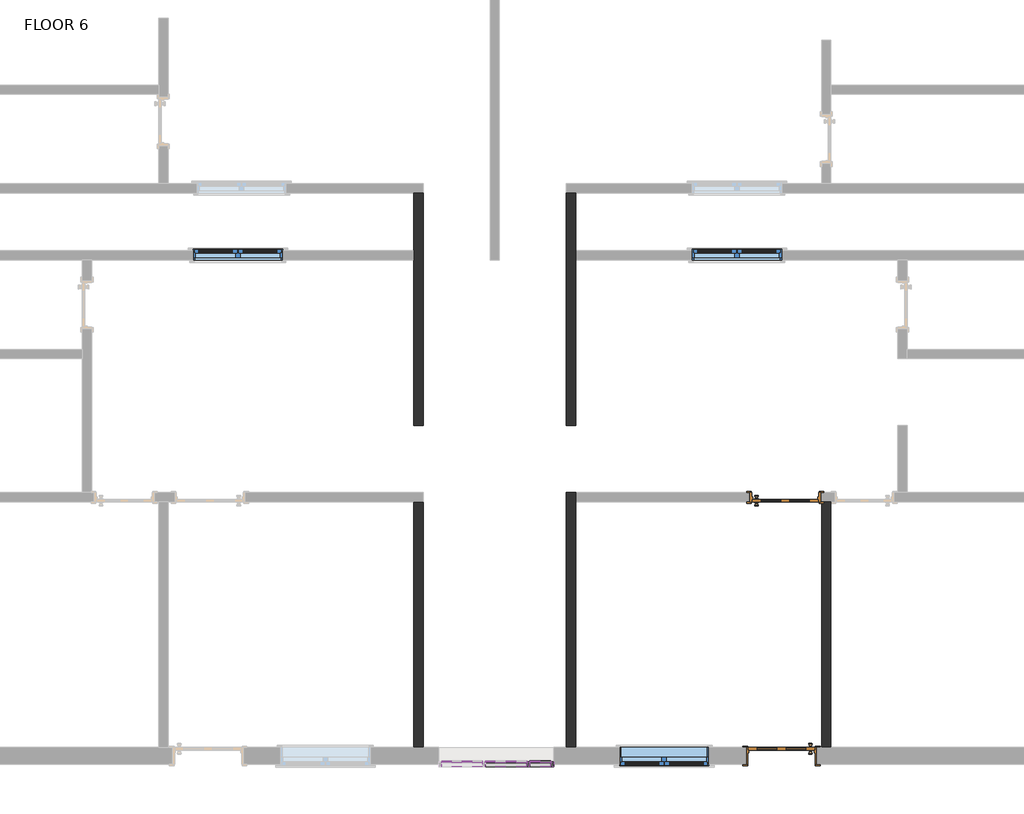
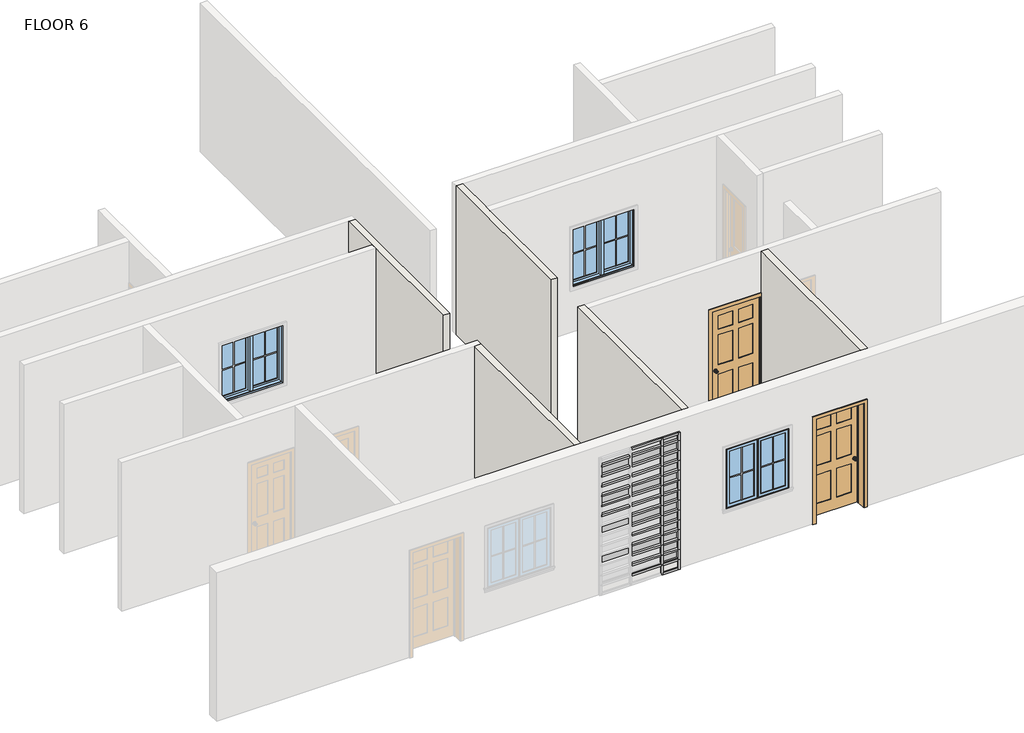
# One storey, part 2 of 4: 63 members, 22 plates, 5 walls, 3 windows, 2 doors.
"""IFC4 building model written with IfcOpenShell, lengths in millimetres."""

from ifc_helpers import new_model, si_unit, frame, origin, place, context, project, spatial, polyline, outline, extrude, faceted_brep, transform, mapped, element, save
from components import door_c610b25b, door_c5239341, member_56b223d9, member_a59c64b1, member_06854975, member_6a7c88b6, member_b8e7570c, member_a67f877f, member_00eacae2, member_ff422208, member_dc11c383, system_panel_glazed_b3845325, system_panel_glazed_23b8b45c, system_panel_glazed_58d257f9, system_panel_glazed_e426d894, system_panel_glazed_822b3193, window_9200f5ac, window_c2c97eee

model = new_model("IFC4")

# Units and contexts
model_context = context("Model", 3, world=origin())
ifc_project = project(units=[si_unit("LENGTHUNIT", "METRE", prefix="MILLI")], contexts=[model_context])

# Site, building, storey
site = spatial("IfcSite", under=ifc_project)
building = spatial("IfcBuilding", under=site)
storey = spatial("IfcBuildingStorey", under=building, Name="FLOOR 6", Elevation=9544.3725604)

# Doors
placement = place(None, origin())
door_shape = door_c610b25b(model_context)
element("IfcDoor", 1, ObjectType="Door-Interior-Single-6_Panel-Wood : 36\" x 84\"", at=placement, inside=storey, context=model_context, shape_type="MappedRepresentation", body=[
    mapped(door_shape, transform((-301.9137331, -4180.7343836, 9544.3725604), x_axis=(1.0, 0.0, 0.0), y_axis=(0.0, 1.0, 0.0), z_axis=(0.0, 0.0, 1.0))),
])
door_2_shape = door_c5239341(model_context)
element("IfcDoor", 2, ObjectType="Door-Interior-Single-6_Panel-Wood : 36\" x 84\"", at=placement, inside=storey, context=model_context, shape_type="MappedRepresentation", body=[
    mapped(door_2_shape, transform((-352.7137331, -7704.9843836, 9544.3725604), x_axis=(-1.0, 0.0, 0.0), y_axis=(0.0, -1.0, 0.0), z_axis=(0.0, 0.0, 1.0))),
])

# Members
member_shape = member_56b223d9(model_context)
element("IfcMember", 3, ObjectType="Rectangular Mullion : 1.5\" x 2.5\" rectangular", at=placement, inside=storey, context=model_context, shape_type="MappedRepresentation", body=[
    mapped(member_shape, transform((-3807.0334597, -7822.4593836, 9544.3725604), x_axis=(1.0, 0.0, 0.0), y_axis=(0.0, -1.0, 0.0), z_axis=(0.0, 0.0, -1.0))),
])
element("IfcMember", 4, ObjectType="Rectangular Mullion : 1.5\" x 2.5\" rectangular", at=placement, inside=storey, context=model_context, shape_type="MappedRepresentation", body=[
    mapped(member_shape, transform((-3807.0334597, -7822.4593836, 9747.5725604), x_axis=(1.0, 0.0, 0.0), y_axis=(0.0, -1.0, 0.0), z_axis=(0.0, 0.0, -1.0))),
])
element("IfcMember", 5, ObjectType="Rectangular Mullion : 1.5\" x 2.5\" rectangular", at=placement, inside=storey, context=model_context, shape_type="MappedRepresentation", body=[
    mapped(member_shape, transform((-3807.0334597, -7822.4593836, 9950.7725604), x_axis=(1.0, 0.0, 0.0), y_axis=(0.0, -1.0, 0.0), z_axis=(0.0, 0.0, -1.0))),
])
element("IfcMember", 6, ObjectType="Rectangular Mullion : 1.5\" x 2.5\" rectangular", at=placement, inside=storey, context=model_context, shape_type="MappedRepresentation", body=[
    mapped(member_shape, transform((-3807.0334597, -7822.4593836, 10153.9725604), x_axis=(1.0, 0.0, 0.0), y_axis=(0.0, -1.0, 0.0), z_axis=(0.0, 0.0, -1.0))),
])
element("IfcMember", 7, ObjectType="Rectangular Mullion : 1.5\" x 2.5\" rectangular", at=placement, inside=storey, context=model_context, shape_type="MappedRepresentation", body=[
    mapped(member_shape, transform((-3807.0334597, -7822.4593836, 10357.1725604), x_axis=(1.0, 0.0, 0.0), y_axis=(0.0, -1.0, 0.0), z_axis=(0.0, 0.0, -1.0))),
])
element("IfcMember", 8, ObjectType="Rectangular Mullion : 1.5\" x 2.5\" rectangular", at=placement, inside=storey, context=model_context, shape_type="MappedRepresentation", body=[
    mapped(member_shape, transform((-3807.0334597, -7822.4593836, 10560.3725604), x_axis=(1.0, 0.0, 0.0), y_axis=(0.0, -1.0, 0.0), z_axis=(0.0, 0.0, -1.0))),
])
element("IfcMember", 9, ObjectType="Rectangular Mullion : 1.5\" x 2.5\" rectangular", at=placement, inside=storey, context=model_context, shape_type="MappedRepresentation", body=[
    mapped(member_shape, transform((-3807.0334597, -7822.4593836, 10763.5725604), x_axis=(1.0, 0.0, 0.0), y_axis=(0.0, -1.0, 0.0), z_axis=(0.0, 0.0, -1.0))),
])
element("IfcMember", 10, ObjectType="Rectangular Mullion : 1.5\" x 2.5\" rectangular", at=placement, inside=storey, context=model_context, shape_type="MappedRepresentation", body=[
    mapped(member_shape, transform((-3807.0334597, -7822.4593836, 10966.7725604), x_axis=(1.0, 0.0, 0.0), y_axis=(0.0, -1.0, 0.0), z_axis=(0.0, 0.0, -1.0))),
])
element("IfcMember", 11, ObjectType="Rectangular Mullion : 1.5\" x 2.5\" rectangular", at=placement, inside=storey, context=model_context, shape_type="MappedRepresentation", body=[
    mapped(member_shape, transform((-3807.0334597, -7822.4593836, 11169.9725604), x_axis=(1.0, 0.0, 0.0), y_axis=(0.0, -1.0, 0.0), z_axis=(0.0, 0.0, -1.0))),
])
element("IfcMember", 12, ObjectType="Rectangular Mullion : 1.5\" x 2.5\" rectangular", at=placement, inside=storey, context=model_context, shape_type="MappedRepresentation", body=[
    mapped(member_shape, transform((-3807.0334597, -7822.4593836, 11373.1725604), x_axis=(1.0, 0.0, 0.0), y_axis=(0.0, -1.0, 0.0), z_axis=(0.0, 0.0, -1.0))),
])
element("IfcMember", 13, ObjectType="Rectangular Mullion : 1.5\" x 2.5\" rectangular", at=placement, inside=storey, context=model_context, shape_type="MappedRepresentation", body=[
    mapped(member_shape, transform((-3807.0334597, -7822.4593836, 11576.3725604), x_axis=(1.0, 0.0, 0.0), y_axis=(0.0, -1.0, 0.0), z_axis=(0.0, 0.0, -1.0))),
])
element("IfcMember", 14, ObjectType="Rectangular Mullion : 1.5\" x 2.5\" rectangular", at=placement, inside=storey, context=model_context, shape_type="MappedRepresentation", body=[
    mapped(member_shape, transform((-3807.0334597, -7822.4593836, 11779.5725604), x_axis=(1.0, 0.0, 0.0), y_axis=(0.0, -1.0, 0.0), z_axis=(0.0, 0.0, -1.0))),
])
element("IfcMember", 15, ObjectType="Rectangular Mullion : 1.5\" x 2.5\" rectangular", at=placement, inside=storey, context=model_context, shape_type="MappedRepresentation", body=[
    mapped(member_shape, transform((-3807.0334597, -7822.4593836, 11982.7725604), x_axis=(1.0, 0.0, 0.0), y_axis=(0.0, -1.0, 0.0), z_axis=(0.0, 0.0, -1.0))),
])
member_2_shape = member_a59c64b1(model_context)
element("IfcMember", 16, ObjectType="Rectangular Mullion : 1.5\" x 2.5\" rectangular", at=placement, inside=storey, context=model_context, shape_type="MappedRepresentation", body=[
    mapped(member_2_shape, transform((-3807.0334597, -7822.4593836, 12185.9725604), x_axis=(1.0, 0.0, 0.0), y_axis=(0.0, -1.0, 0.0), z_axis=(0.0, 0.0, -1.0))),
])
member_3_shape = member_06854975(model_context)
element("IfcMember", 17, ObjectType="Rectangular Mullion : 1.5\" x 2.5\" rectangular", at=placement, inside=storey, context=model_context, shape_type="MappedRepresentation", body=[
    mapped(member_3_shape, transform((-3499.7513929, -7822.4593836, 12351.7551755), x_axis=(0.0, 0.0, 1.0), y_axis=(0.0, -1.0, 0.0), z_axis=(1.0, 0.0, 0.0))),
])
member_4_shape = member_6a7c88b6(model_context)
element("IfcMember", 18, ObjectType="Rectangular Mullion : 1.5\" x 2.5\" rectangular", at=placement, inside=storey, context=model_context, shape_type="MappedRepresentation", body=[
    mapped(member_4_shape, transform((-4435.6834597, -7822.4593836, 11169.9725604), x_axis=(0.0, 0.0, 1.0), y_axis=(0.0, -1.0, 0.0), z_axis=(1.0, 0.0, 0.0))),
])
element("IfcMember", 19, ObjectType="Rectangular Mullion : 1.5\" x 2.5\" rectangular", at=placement, inside=storey, context=model_context, shape_type="MappedRepresentation", body=[
    mapped(member_4_shape, transform((-4435.6834597, -7822.4593836, 11373.1725604), x_axis=(0.0, 0.0, 1.0), y_axis=(0.0, -1.0, 0.0), z_axis=(1.0, 0.0, 0.0))),
])
element("IfcMember", 20, ObjectType="Rectangular Mullion : 1.5\" x 2.5\" rectangular", at=placement, inside=storey, context=model_context, shape_type="MappedRepresentation", body=[
    mapped(member_4_shape, transform((-4435.6834597, -7822.4593836, 11576.3725604), x_axis=(0.0, 0.0, 1.0), y_axis=(0.0, -1.0, 0.0), z_axis=(1.0, 0.0, 0.0))),
])
element("IfcMember", 21, ObjectType="Rectangular Mullion : 1.5\" x 2.5\" rectangular", at=placement, inside=storey, context=model_context, shape_type="MappedRepresentation", body=[
    mapped(member_4_shape, transform((-4435.6834597, -7822.4593836, 11779.5725604), x_axis=(0.0, 0.0, 1.0), y_axis=(0.0, -1.0, 0.0), z_axis=(1.0, 0.0, 0.0))),
])
element("IfcMember", 22, ObjectType="Rectangular Mullion : 1.5\" x 2.5\" rectangular", at=placement, inside=storey, context=model_context, shape_type="MappedRepresentation", body=[
    mapped(member_4_shape, transform((-4435.6834597, -7822.4593836, 11982.7725604), x_axis=(0.0, 0.0, 1.0), y_axis=(0.0, -1.0, 0.0), z_axis=(1.0, 0.0, 0.0))),
])
element("IfcMember", 23, ObjectType="Rectangular Mullion : 1.5\" x 2.5\" rectangular", at=placement, inside=storey, context=model_context, shape_type="MappedRepresentation", body=[
    mapped(member_4_shape, transform((-4435.6834597, -7822.4593836, 12185.9725604), x_axis=(0.0, 0.0, 1.0), y_axis=(0.0, -1.0, 0.0), z_axis=(1.0, 0.0, 0.0))),
])
member_5_shape = member_b8e7570c(model_context)
element("IfcMember", 24, ObjectType="Rectangular Mullion : 1.5\" x 2.5\" rectangular", at=placement, inside=storey, context=model_context, shape_type="MappedRepresentation", body=[
    mapped(member_5_shape, transform((-3826.0834597, -7822.4593836, 9747.5725604), x_axis=(0.0, 0.0, 1.0), y_axis=(0.0, -1.0, 0.0), z_axis=(1.0, 0.0, 0.0))),
])
element("IfcMember", 25, ObjectType="Rectangular Mullion : 1.5\" x 2.5\" rectangular", at=placement, inside=storey, context=model_context, shape_type="MappedRepresentation", body=[
    mapped(member_5_shape, transform((-3826.0834597, -7822.4593836, 9950.7725604), x_axis=(0.0, 0.0, 1.0), y_axis=(0.0, -1.0, 0.0), z_axis=(1.0, 0.0, 0.0))),
])
element("IfcMember", 26, ObjectType="Rectangular Mullion : 1.5\" x 2.5\" rectangular", at=placement, inside=storey, context=model_context, shape_type="MappedRepresentation", body=[
    mapped(member_5_shape, transform((-3826.0834597, -7822.4593836, 10153.9725604), x_axis=(0.0, 0.0, 1.0), y_axis=(0.0, -1.0, 0.0), z_axis=(1.0, 0.0, 0.0))),
])
element("IfcMember", 27, ObjectType="Rectangular Mullion : 1.5\" x 2.5\" rectangular", at=placement, inside=storey, context=model_context, shape_type="MappedRepresentation", body=[
    mapped(member_5_shape, transform((-3826.0834597, -7822.4593836, 10357.1725604), x_axis=(0.0, 0.0, 1.0), y_axis=(0.0, -1.0, 0.0), z_axis=(1.0, 0.0, 0.0))),
])
element("IfcMember", 28, ObjectType="Rectangular Mullion : 1.5\" x 2.5\" rectangular", at=placement, inside=storey, context=model_context, shape_type="MappedRepresentation", body=[
    mapped(member_5_shape, transform((-3826.0834597, -7822.4593836, 10560.3725604), x_axis=(0.0, 0.0, 1.0), y_axis=(0.0, -1.0, 0.0), z_axis=(1.0, 0.0, 0.0))),
])
element("IfcMember", 29, ObjectType="Rectangular Mullion : 1.5\" x 2.5\" rectangular", at=placement, inside=storey, context=model_context, shape_type="MappedRepresentation", body=[
    mapped(member_5_shape, transform((-3826.0834597, -7822.4593836, 10763.5725604), x_axis=(0.0, 0.0, 1.0), y_axis=(0.0, -1.0, 0.0), z_axis=(1.0, 0.0, 0.0))),
])
element("IfcMember", 30, ObjectType="Rectangular Mullion : 1.5\" x 2.5\" rectangular", at=placement, inside=storey, context=model_context, shape_type="MappedRepresentation", body=[
    mapped(member_5_shape, transform((-3826.0834597, -7822.4593836, 10966.7725604), x_axis=(0.0, 0.0, 1.0), y_axis=(0.0, -1.0, 0.0), z_axis=(1.0, 0.0, 0.0))),
])
element("IfcMember", 31, ObjectType="Rectangular Mullion : 1.5\" x 2.5\" rectangular", at=placement, inside=storey, context=model_context, shape_type="MappedRepresentation", body=[
    mapped(member_5_shape, transform((-3826.0834597, -7822.4593836, 11169.9725604), x_axis=(0.0, 0.0, 1.0), y_axis=(0.0, -1.0, 0.0), z_axis=(1.0, 0.0, 0.0))),
])
element("IfcMember", 32, ObjectType="Rectangular Mullion : 1.5\" x 2.5\" rectangular", at=placement, inside=storey, context=model_context, shape_type="MappedRepresentation", body=[
    mapped(member_5_shape, transform((-3826.0834597, -7822.4593836, 11373.1725604), x_axis=(0.0, 0.0, 1.0), y_axis=(0.0, -1.0, 0.0), z_axis=(1.0, 0.0, 0.0))),
])
element("IfcMember", 33, ObjectType="Rectangular Mullion : 1.5\" x 2.5\" rectangular", at=placement, inside=storey, context=model_context, shape_type="MappedRepresentation", body=[
    mapped(member_5_shape, transform((-3826.0834597, -7822.4593836, 11576.3725604), x_axis=(0.0, 0.0, 1.0), y_axis=(0.0, -1.0, 0.0), z_axis=(1.0, 0.0, 0.0))),
])
element("IfcMember", 34, ObjectType="Rectangular Mullion : 1.5\" x 2.5\" rectangular", at=placement, inside=storey, context=model_context, shape_type="MappedRepresentation", body=[
    mapped(member_5_shape, transform((-3826.0834597, -7822.4593836, 11779.5725604), x_axis=(0.0, 0.0, 1.0), y_axis=(0.0, -1.0, 0.0), z_axis=(1.0, 0.0, 0.0))),
])
element("IfcMember", 35, ObjectType="Rectangular Mullion : 1.5\" x 2.5\" rectangular", at=placement, inside=storey, context=model_context, shape_type="MappedRepresentation", body=[
    mapped(member_5_shape, transform((-3826.0834597, -7822.4593836, 11982.7725604), x_axis=(0.0, 0.0, 1.0), y_axis=(0.0, -1.0, 0.0), z_axis=(1.0, 0.0, 0.0))),
])
element("IfcMember", 36, ObjectType="Rectangular Mullion : 1.5\" x 2.5\" rectangular", at=placement, inside=storey, context=model_context, shape_type="MappedRepresentation", body=[
    mapped(member_5_shape, transform((-3826.0834597, -7822.4593836, 12185.9725604), x_axis=(0.0, 0.0, 1.0), y_axis=(0.0, -1.0, 0.0), z_axis=(1.0, 0.0, 0.0))),
])
member_6_shape = member_a67f877f(model_context)
element("IfcMember", 37, ObjectType="Rectangular Mullion : 1.5\" x 2.5\" rectangular", at=placement, inside=storey, context=model_context, shape_type="MappedRepresentation", body=[
    mapped(member_6_shape, transform((-3826.0834597, -7822.4593836, 12351.7551755), x_axis=(0.0, 0.0, 1.0), y_axis=(0.0, -1.0, 0.0), z_axis=(1.0, 0.0, 0.0))),
])
element("IfcMember", 38, ObjectType="Rectangular Mullion : 1.5\" x 2.5\" rectangular", at=placement, inside=storey, context=model_context, shape_type="MappedRepresentation", body=[
    mapped(member_3_shape, transform((-3787.9834597, -7822.4593836, 9544.3725604), x_axis=(0.0, 0.0, -1.0), y_axis=(0.0, -1.0, 0.0), z_axis=(-1.0, 0.0, 0.0))),
])
member_7_shape = member_00eacae2(model_context)
element("IfcMember", 39, ObjectType="Rectangular Mullion : 1.5\" x 2.5\" rectangular", at=placement, inside=storey, context=model_context, shape_type="MappedRepresentation", body=[
    mapped(member_7_shape, transform((-3499.7513929, -7822.4593836, 9747.5725604), x_axis=(0.0, 0.0, 1.0), y_axis=(0.0, -1.0, 0.0), z_axis=(1.0, 0.0, 0.0))),
])
element("IfcMember", 40, ObjectType="Rectangular Mullion : 1.5\" x 2.5\" rectangular", at=placement, inside=storey, context=model_context, shape_type="MappedRepresentation", body=[
    mapped(member_7_shape, transform((-3499.7513929, -7822.4593836, 9950.7725604), x_axis=(0.0, 0.0, 1.0), y_axis=(0.0, -1.0, 0.0), z_axis=(1.0, 0.0, 0.0))),
])
element("IfcMember", 41, ObjectType="Rectangular Mullion : 1.5\" x 2.5\" rectangular", at=placement, inside=storey, context=model_context, shape_type="MappedRepresentation", body=[
    mapped(member_7_shape, transform((-3499.7513929, -7822.4593836, 10153.9725604), x_axis=(0.0, 0.0, 1.0), y_axis=(0.0, -1.0, 0.0), z_axis=(1.0, 0.0, 0.0))),
])
element("IfcMember", 42, ObjectType="Rectangular Mullion : 1.5\" x 2.5\" rectangular", at=placement, inside=storey, context=model_context, shape_type="MappedRepresentation", body=[
    mapped(member_7_shape, transform((-3499.7513929, -7822.4593836, 10357.1725604), x_axis=(0.0, 0.0, 1.0), y_axis=(0.0, -1.0, 0.0), z_axis=(1.0, 0.0, 0.0))),
])
element("IfcMember", 43, ObjectType="Rectangular Mullion : 1.5\" x 2.5\" rectangular", at=placement, inside=storey, context=model_context, shape_type="MappedRepresentation", body=[
    mapped(member_7_shape, transform((-3499.7513929, -7822.4593836, 10560.3725604), x_axis=(0.0, 0.0, 1.0), y_axis=(0.0, -1.0, 0.0), z_axis=(1.0, 0.0, 0.0))),
])
element("IfcMember", 44, ObjectType="Rectangular Mullion : 1.5\" x 2.5\" rectangular", at=placement, inside=storey, context=model_context, shape_type="MappedRepresentation", body=[
    mapped(member_7_shape, transform((-3499.7513929, -7822.4593836, 10763.5725604), x_axis=(0.0, 0.0, 1.0), y_axis=(0.0, -1.0, 0.0), z_axis=(1.0, 0.0, 0.0))),
])
element("IfcMember", 45, ObjectType="Rectangular Mullion : 1.5\" x 2.5\" rectangular", at=placement, inside=storey, context=model_context, shape_type="MappedRepresentation", body=[
    mapped(member_7_shape, transform((-3499.7513929, -7822.4593836, 10966.7725604), x_axis=(0.0, 0.0, 1.0), y_axis=(0.0, -1.0, 0.0), z_axis=(1.0, 0.0, 0.0))),
])
element("IfcMember", 46, ObjectType="Rectangular Mullion : 1.5\" x 2.5\" rectangular", at=placement, inside=storey, context=model_context, shape_type="MappedRepresentation", body=[
    mapped(member_7_shape, transform((-3499.7513929, -7822.4593836, 11169.9725604), x_axis=(0.0, 0.0, 1.0), y_axis=(0.0, -1.0, 0.0), z_axis=(1.0, 0.0, 0.0))),
])
element("IfcMember", 47, ObjectType="Rectangular Mullion : 1.5\" x 2.5\" rectangular", at=placement, inside=storey, context=model_context, shape_type="MappedRepresentation", body=[
    mapped(member_7_shape, transform((-3499.7513929, -7822.4593836, 11373.1725604), x_axis=(0.0, 0.0, 1.0), y_axis=(0.0, -1.0, 0.0), z_axis=(1.0, 0.0, 0.0))),
])
element("IfcMember", 48, ObjectType="Rectangular Mullion : 1.5\" x 2.5\" rectangular", at=placement, inside=storey, context=model_context, shape_type="MappedRepresentation", body=[
    mapped(member_7_shape, transform((-3499.7513929, -7822.4593836, 11576.3725604), x_axis=(0.0, 0.0, 1.0), y_axis=(0.0, -1.0, 0.0), z_axis=(1.0, 0.0, 0.0))),
])
element("IfcMember", 49, ObjectType="Rectangular Mullion : 1.5\" x 2.5\" rectangular", at=placement, inside=storey, context=model_context, shape_type="MappedRepresentation", body=[
    mapped(member_7_shape, transform((-3499.7513929, -7822.4593836, 11779.5725604), x_axis=(0.0, 0.0, 1.0), y_axis=(0.0, -1.0, 0.0), z_axis=(1.0, 0.0, 0.0))),
])
element("IfcMember", 50, ObjectType="Rectangular Mullion : 1.5\" x 2.5\" rectangular", at=placement, inside=storey, context=model_context, shape_type="MappedRepresentation", body=[
    mapped(member_7_shape, transform((-3499.7513929, -7822.4593836, 11982.7725604), x_axis=(0.0, 0.0, 1.0), y_axis=(0.0, -1.0, 0.0), z_axis=(1.0, 0.0, 0.0))),
])
element("IfcMember", 51, ObjectType="Rectangular Mullion : 1.5\" x 2.5\" rectangular", at=placement, inside=storey, context=model_context, shape_type="MappedRepresentation", body=[
    mapped(member_7_shape, transform((-3499.7513929, -7822.4593836, 12185.9725604), x_axis=(0.0, 0.0, 1.0), y_axis=(0.0, -1.0, 0.0), z_axis=(1.0, 0.0, 0.0))),
])
member_8_shape = member_ff422208(model_context)
element("IfcMember", 52, ObjectType="Rectangular Mullion : 1.5\" x 2.5\" rectangular", at=placement, inside=storey, context=model_context, shape_type="MappedRepresentation", body=[
    mapped(member_8_shape, transform((-3461.6513929, -7822.4593836, 9544.3725604), x_axis=(1.0, 0.0, 0.0), y_axis=(0.0, -1.0, 0.0), z_axis=(0.0, 0.0, -1.0))),
])
element("IfcMember", 53, ObjectType="Rectangular Mullion : 1.5\" x 2.5\" rectangular", at=placement, inside=storey, context=model_context, shape_type="MappedRepresentation", body=[
    mapped(member_8_shape, transform((-3461.6513929, -7822.4593836, 9747.5725604), x_axis=(1.0, 0.0, 0.0), y_axis=(0.0, -1.0, 0.0), z_axis=(0.0, 0.0, -1.0))),
])
element("IfcMember", 54, ObjectType="Rectangular Mullion : 1.5\" x 2.5\" rectangular", at=placement, inside=storey, context=model_context, shape_type="MappedRepresentation", body=[
    mapped(member_8_shape, transform((-3461.6513929, -7822.4593836, 9950.7725604), x_axis=(1.0, 0.0, 0.0), y_axis=(0.0, -1.0, 0.0), z_axis=(0.0, 0.0, -1.0))),
])
element("IfcMember", 55, ObjectType="Rectangular Mullion : 1.5\" x 2.5\" rectangular", at=placement, inside=storey, context=model_context, shape_type="MappedRepresentation", body=[
    mapped(member_8_shape, transform((-3461.6513929, -7822.4593836, 10153.9725604), x_axis=(1.0, 0.0, 0.0), y_axis=(0.0, -1.0, 0.0), z_axis=(0.0, 0.0, -1.0))),
])
element("IfcMember", 56, ObjectType="Rectangular Mullion : 1.5\" x 2.5\" rectangular", at=placement, inside=storey, context=model_context, shape_type="MappedRepresentation", body=[
    mapped(member_8_shape, transform((-3461.6513929, -7822.4593836, 10357.1725604), x_axis=(1.0, 0.0, 0.0), y_axis=(0.0, -1.0, 0.0), z_axis=(0.0, 0.0, -1.0))),
])
element("IfcMember", 57, ObjectType="Rectangular Mullion : 1.5\" x 2.5\" rectangular", at=placement, inside=storey, context=model_context, shape_type="MappedRepresentation", body=[
    mapped(member_8_shape, transform((-3461.6513929, -7822.4593836, 10560.3725604), x_axis=(1.0, 0.0, 0.0), y_axis=(0.0, -1.0, 0.0), z_axis=(0.0, 0.0, -1.0))),
])
element("IfcMember", 58, ObjectType="Rectangular Mullion : 1.5\" x 2.5\" rectangular", at=placement, inside=storey, context=model_context, shape_type="MappedRepresentation", body=[
    mapped(member_8_shape, transform((-3461.6513929, -7822.4593836, 10763.5725604), x_axis=(1.0, 0.0, 0.0), y_axis=(0.0, -1.0, 0.0), z_axis=(0.0, 0.0, -1.0))),
])
element("IfcMember", 59, ObjectType="Rectangular Mullion : 1.5\" x 2.5\" rectangular", at=placement, inside=storey, context=model_context, shape_type="MappedRepresentation", body=[
    mapped(member_8_shape, transform((-3461.6513929, -7822.4593836, 10966.7725604), x_axis=(1.0, 0.0, 0.0), y_axis=(0.0, -1.0, 0.0), z_axis=(0.0, 0.0, -1.0))),
])
element("IfcMember", 60, ObjectType="Rectangular Mullion : 1.5\" x 2.5\" rectangular", at=placement, inside=storey, context=model_context, shape_type="MappedRepresentation", body=[
    mapped(member_8_shape, transform((-3461.6513929, -7822.4593836, 11169.9725604), x_axis=(1.0, 0.0, 0.0), y_axis=(0.0, -1.0, 0.0), z_axis=(0.0, 0.0, -1.0))),
])
element("IfcMember", 61, ObjectType="Rectangular Mullion : 1.5\" x 2.5\" rectangular", at=placement, inside=storey, context=model_context, shape_type="MappedRepresentation", body=[
    mapped(member_8_shape, transform((-3461.6513929, -7822.4593836, 11373.1725604), x_axis=(1.0, 0.0, 0.0), y_axis=(0.0, -1.0, 0.0), z_axis=(0.0, 0.0, -1.0))),
])
element("IfcMember", 62, ObjectType="Rectangular Mullion : 1.5\" x 2.5\" rectangular", at=placement, inside=storey, context=model_context, shape_type="MappedRepresentation", body=[
    mapped(member_8_shape, transform((-3461.6513929, -7822.4593836, 11576.3725604), x_axis=(1.0, 0.0, 0.0), y_axis=(0.0, -1.0, 0.0), z_axis=(0.0, 0.0, -1.0))),
])
element("IfcMember", 63, ObjectType="Rectangular Mullion : 1.5\" x 2.5\" rectangular", at=placement, inside=storey, context=model_context, shape_type="MappedRepresentation", body=[
    mapped(member_8_shape, transform((-3461.6513929, -7822.4593836, 11779.5725604), x_axis=(1.0, 0.0, 0.0), y_axis=(0.0, -1.0, 0.0), z_axis=(0.0, 0.0, -1.0))),
])
element("IfcMember", 64, ObjectType="Rectangular Mullion : 1.5\" x 2.5\" rectangular", at=placement, inside=storey, context=model_context, shape_type="MappedRepresentation", body=[
    mapped(member_8_shape, transform((-3461.6513929, -7822.4593836, 11982.7725604), x_axis=(1.0, 0.0, 0.0), y_axis=(0.0, -1.0, 0.0), z_axis=(0.0, 0.0, -1.0))),
])
member_9_shape = member_dc11c383(model_context)
element("IfcMember", 65, ObjectType="Rectangular Mullion : 1.5\" x 2.5\" rectangular", at=placement, inside=storey, context=model_context, shape_type="MappedRepresentation", body=[
    mapped(member_9_shape, transform((-3461.6513929, -7822.4593836, 12185.9725604), x_axis=(1.0, 0.0, 0.0), y_axis=(0.0, -1.0, 0.0), z_axis=(0.0, 0.0, -1.0))),
])

# Plates
system_panel_glazed_shape = system_panel_glazed_b3845325(model_context)
element("IfcPlate", 66, ObjectType="System Panel : Glazed", at=placement, inside=storey, context=model_context, shape_type="MappedRepresentation", body=[
    mapped(system_panel_glazed_shape, transform((-4711.9084599, -7822.4593836, 10173.0225604), x_axis=(1.0, 0.0, 0.0), y_axis=(0.0, 1.0, 0.0), z_axis=(0.0, 0.0, 1.0))),
])
element("IfcPlate", 67, ObjectType="System Panel : Glazed", at=placement, inside=storey, context=model_context, shape_type="MappedRepresentation", body=[
    mapped(system_panel_glazed_shape, transform((-4711.9084599, -7822.4593836, 10782.6225604), x_axis=(1.0, 0.0, 0.0), y_axis=(0.0, 1.0, 0.0), z_axis=(0.0, 0.0, 1.0))),
])
element("IfcPlate", 68, ObjectType="System Panel : Glazed", at=placement, inside=storey, context=model_context, shape_type="MappedRepresentation", body=[
    mapped(system_panel_glazed_shape, transform((-4711.9084599, -7822.4593836, 11392.2225604), x_axis=(1.0, 0.0, 0.0), y_axis=(0.0, 1.0, 0.0), z_axis=(0.0, 0.0, 1.0))),
])
element("IfcPlate", 69, ObjectType="System Panel : Glazed", at=placement, inside=storey, context=model_context, shape_type="MappedRepresentation", body=[
    mapped(system_panel_glazed_shape, transform((-4711.9084599, -7822.4593836, 12001.8225604), x_axis=(1.0, 0.0, 0.0), y_axis=(0.0, 1.0, 0.0), z_axis=(0.0, 0.0, 1.0))),
])
system_panel_glazed_2_shape = system_panel_glazed_23b8b45c(model_context)
element("IfcPlate", 70, ObjectType="System Panel : Glazed", at=placement, inside=storey, context=model_context, shape_type="MappedRepresentation", body=[
    mapped(system_panel_glazed_2_shape, transform((-4111.8334597, -7822.4593836, 10173.0225604), x_axis=(1.0, 0.0, 0.0), y_axis=(0.0, 1.0, 0.0), z_axis=(0.0, 0.0, 1.0))),
])
element("IfcPlate", 71, ObjectType="System Panel : Glazed", at=placement, inside=storey, context=model_context, shape_type="MappedRepresentation", body=[
    mapped(system_panel_glazed_2_shape, transform((-4111.8334597, -7822.4593836, 10782.6225604), x_axis=(1.0, 0.0, 0.0), y_axis=(0.0, 1.0, 0.0), z_axis=(0.0, 0.0, 1.0))),
])
element("IfcPlate", 72, ObjectType="System Panel : Glazed", at=placement, inside=storey, context=model_context, shape_type="MappedRepresentation", body=[
    mapped(system_panel_glazed_2_shape, transform((-4111.8334597, -7822.4593836, 11392.2225604), x_axis=(1.0, 0.0, 0.0), y_axis=(0.0, 1.0, 0.0), z_axis=(0.0, 0.0, 1.0))),
])
element("IfcPlate", 73, ObjectType="System Panel : Glazed", at=placement, inside=storey, context=model_context, shape_type="MappedRepresentation", body=[
    mapped(system_panel_glazed_2_shape, transform((-4111.8334597, -7822.4593836, 12001.8225604), x_axis=(1.0, 0.0, 0.0), y_axis=(0.0, 1.0, 0.0), z_axis=(0.0, 0.0, 1.0))),
])
system_panel_glazed_3_shape = system_panel_glazed_58d257f9(model_context)
element("IfcPlate", 74, ObjectType="System Panel : Glazed", at=placement, inside=storey, context=model_context, shape_type="MappedRepresentation", body=[
    mapped(system_panel_glazed_3_shape, transform((-3643.8674263, -7822.4593836, 9582.4725604), x_axis=(1.0, 0.0, 0.0), y_axis=(0.0, 1.0, 0.0), z_axis=(0.0, 0.0, 1.0))),
])
system_panel_glazed_4_shape = system_panel_glazed_e426d894(model_context)
element("IfcPlate", 75, ObjectType="System Panel : Glazed", at=placement, inside=storey, context=model_context, shape_type="MappedRepresentation", body=[
    mapped(system_panel_glazed_4_shape, transform((-3643.8674263, -7822.4593836, 9766.6225604), x_axis=(1.0, 0.0, 0.0), y_axis=(0.0, 1.0, 0.0), z_axis=(0.0, 0.0, 1.0))),
])
element("IfcPlate", 76, ObjectType="System Panel : Glazed", at=placement, inside=storey, context=model_context, shape_type="MappedRepresentation", body=[
    mapped(system_panel_glazed_4_shape, transform((-3643.8674263, -7822.4593836, 9969.8225604), x_axis=(1.0, 0.0, 0.0), y_axis=(0.0, 1.0, 0.0), z_axis=(0.0, 0.0, 1.0))),
])
element("IfcPlate", 77, ObjectType="System Panel : Glazed", at=placement, inside=storey, context=model_context, shape_type="MappedRepresentation", body=[
    mapped(system_panel_glazed_4_shape, transform((-3643.8674263, -7822.4593836, 10376.2225604), x_axis=(1.0, 0.0, 0.0), y_axis=(0.0, 1.0, 0.0), z_axis=(0.0, 0.0, 1.0))),
])
element("IfcPlate", 78, ObjectType="System Panel : Glazed", at=placement, inside=storey, context=model_context, shape_type="MappedRepresentation", body=[
    mapped(system_panel_glazed_4_shape, transform((-3643.8674263, -7822.4593836, 10579.4225604), x_axis=(1.0, 0.0, 0.0), y_axis=(0.0, 1.0, 0.0), z_axis=(0.0, 0.0, 1.0))),
])
element("IfcPlate", 79, ObjectType="System Panel : Glazed", at=placement, inside=storey, context=model_context, shape_type="MappedRepresentation", body=[
    mapped(system_panel_glazed_4_shape, transform((-3643.8674263, -7822.4593836, 10985.8225604), x_axis=(1.0, 0.0, 0.0), y_axis=(0.0, 1.0, 0.0), z_axis=(0.0, 0.0, 1.0))),
])
element("IfcPlate", 80, ObjectType="System Panel : Glazed", at=placement, inside=storey, context=model_context, shape_type="MappedRepresentation", body=[
    mapped(system_panel_glazed_4_shape, transform((-3643.8674263, -7822.4593836, 11189.0225604), x_axis=(1.0, 0.0, 0.0), y_axis=(0.0, 1.0, 0.0), z_axis=(0.0, 0.0, 1.0))),
])
element("IfcPlate", 81, ObjectType="System Panel : Glazed", at=placement, inside=storey, context=model_context, shape_type="MappedRepresentation", body=[
    mapped(system_panel_glazed_4_shape, transform((-3643.8674263, -7822.4593836, 11595.4225604), x_axis=(1.0, 0.0, 0.0), y_axis=(0.0, 1.0, 0.0), z_axis=(0.0, 0.0, 1.0))),
])
element("IfcPlate", 82, ObjectType="System Panel : Glazed", at=placement, inside=storey, context=model_context, shape_type="MappedRepresentation", body=[
    mapped(system_panel_glazed_4_shape, transform((-3643.8674263, -7822.4593836, 11798.6225604), x_axis=(1.0, 0.0, 0.0), y_axis=(0.0, 1.0, 0.0), z_axis=(0.0, 0.0, 1.0))),
])
element("IfcPlate", 83, ObjectType="System Panel : Glazed", at=placement, inside=storey, context=model_context, shape_type="MappedRepresentation", body=[
    mapped(system_panel_glazed_4_shape, transform((-3643.8674263, -7822.4593836, 10173.0225604), x_axis=(1.0, 0.0, 0.0), y_axis=(0.0, 1.0, 0.0), z_axis=(0.0, 0.0, 1.0))),
])
element("IfcPlate", 84, ObjectType="System Panel : Glazed", at=placement, inside=storey, context=model_context, shape_type="MappedRepresentation", body=[
    mapped(system_panel_glazed_4_shape, transform((-3643.8674263, -7822.4593836, 10782.6225604), x_axis=(1.0, 0.0, 0.0), y_axis=(0.0, 1.0, 0.0), z_axis=(0.0, 0.0, 1.0))),
])
element("IfcPlate", 85, ObjectType="System Panel : Glazed", at=placement, inside=storey, context=model_context, shape_type="MappedRepresentation", body=[
    mapped(system_panel_glazed_4_shape, transform((-3643.8674263, -7822.4593836, 11392.2225604), x_axis=(1.0, 0.0, 0.0), y_axis=(0.0, 1.0, 0.0), z_axis=(0.0, 0.0, 1.0))),
])
element("IfcPlate", 86, ObjectType="System Panel : Glazed", at=placement, inside=storey, context=model_context, shape_type="MappedRepresentation", body=[
    mapped(system_panel_glazed_4_shape, transform((-3643.8674263, -7822.4593836, 12001.8225604), x_axis=(1.0, 0.0, 0.0), y_axis=(0.0, 1.0, 0.0), z_axis=(0.0, 0.0, 1.0))),
])
system_panel_glazed_5_shape = system_panel_glazed_822b3193(model_context)
element("IfcPlate", 87, ObjectType="System Panel : Glazed", at=placement, inside=storey, context=model_context, shape_type="MappedRepresentation", body=[
    mapped(system_panel_glazed_5_shape, transform((-3643.8674263, -7822.4593836, 12205.0225604), x_axis=(1.0, 0.0, 0.0), y_axis=(0.0, 1.0, 0.0), z_axis=(0.0, 0.0, 1.0))),
])

# Walls
element("IfcWall", 88, ObjectType="Inner Wall 5\"", at=placement, inside=storey, context=model_context, shape_type="Brep", body=[
    faceted_brep([(-5369.2137331, -24.6593836, 9544.3725604), (-5369.2137331, -812.0593836, 9544.3725604), (-5369.2137331, -939.0593836, 9544.3725604), (-5369.2137331, -3199.6593836, 9544.3725604), (-5369.2137331, -3199.6593836, 12592.3725604), (-5369.2137331, -939.0593836, 12592.3725604), (-5369.2137331, -812.0593836, 12592.3725604), (-5369.2137331, -24.6593836, 12592.3725604), (-5242.2137331, -24.6593836, 9544.3725604), (-5242.2137331, -24.6593836, 12592.3725604), (-5242.2137331, -3199.6593836, 12592.3725604), (-5242.2137331, -3199.6593836, 9544.3725604)], [[[0, 1, 2, 3, 4, 5, 6, 7]], [[8, 9, 10, 11]], [[3, 2, 1, 0, 8, 11]], [[4, 3, 11, 10]], [[7, 6, 5, 4, 10, 9]], [[0, 7, 9, 8]]]),
])
element("IfcWall", 89, ObjectType="Inner Wall 5\"", at=placement, inside=storey, context=model_context, shape_type="Brep", body=[
    faceted_brep([(-3286.4137331, -24.6593836, 9544.3725604), (-3286.4137331, -3199.6593836, 9544.3725604), (-3286.4137331, -3199.6593836, 12592.3725604), (-3286.4137331, -24.6593836, 12592.3725604), (-3159.4137331, -24.6593836, 9544.3725604), (-3159.4137331, -24.6593836, 12592.3725604), (-3159.4137331, -812.0593836, 12592.3725604), (-3159.4137331, -939.0593836, 12592.3725604), (-3159.4137331, -3199.6593836, 12592.3725604), (-3159.4137331, -3199.6593836, 9544.3725604), (-3159.4137331, -939.0593836, 9544.3725604), (-3159.4137331, -812.0593836, 9544.3725604)], [[[0, 1, 2, 3]], [[4, 5, 6, 7, 8, 9, 10, 11]], [[1, 0, 4, 11, 10, 9]], [[2, 1, 9, 8]], [[3, 2, 8, 7, 6, 5]], [[0, 3, 5, 4]]]),
])
element("IfcWall", 90, ObjectType="Inner Wall 5\"", at=placement, inside=storey, context=model_context, shape_type="SweptSolid", body=[
    extrude(outline(polyline([(-5242.2137331, -4241.0593836), (-5242.2137331, -7593.8593836), (-5369.2137331, -7593.8593836), (-5369.2137331, -4241.0593836), (-5242.2137331, -4241.0593836)])), frame((0.0, 0.0, 9544.3725604), z_axis=(0.0, 0.0, 1.0), x_axis=(1.0, 0.0, 0.0)), (0.0, 0.0, 1.0), 3048.0),
])
element("IfcWall", 91, ObjectType="Inner Wall 5\"", at=placement, inside=storey, context=model_context, shape_type="Brep", body=[
    faceted_brep([(-3159.4137331, -7593.8593836, 9544.3725604), (-3159.4137331, -4241.0593836, 9544.3725604), (-3159.4137331, -4114.0593836, 9544.3725604), (-3159.4137331, -4114.0593836, 12592.3725604), (-3159.4137331, -4241.0593836, 12592.3725604), (-3159.4137331, -7593.8593836, 12592.3725604), (-3286.4137331, -7593.8593836, 9544.3725604), (-3286.4137331, -7593.8593836, 12592.3725604), (-3286.4137331, -4114.0593836, 12592.3725604), (-3286.4137331, -4114.0593836, 9544.3725604)], [[[0, 1, 2, 3, 4, 5]], [[6, 7, 8, 9]], [[2, 1, 0, 6, 9]], [[5, 4, 3, 8, 7]], [[0, 5, 7, 6]], [[3, 2, 9, 8]]]),
])
element("IfcWall", 92, ObjectType="Inner Wall 5\"", at=placement, inside=storey, context=model_context, shape_type="SweptSolid", body=[
    extrude(outline(polyline([(320.3862669, -4241.0593836), (320.3862669, -7593.8593836), (193.3862669, -7593.8593836), (193.3862669, -4241.0593836), (320.3862669, -4241.0593836)])), frame((0.0, 0.0, 9544.3725604), z_axis=(0.0, 0.0, 1.0), x_axis=(1.0, 0.0, 0.0)), (0.0, 0.0, 1.0), 3048.0),
])

# Windows
window_shape = window_9200f5ac(model_context)
element("IfcWindow", 93, ObjectType="Window-Casement-Double : 48\" x 48\"", at=placement, inside=storey, context=model_context, shape_type="MappedRepresentation", body=[
    mapped(window_shape, transform((-1952.9137331, -7708.1593836, 9544.3725604), x_axis=(-1.0, 0.0, 0.0), y_axis=(0.0, -1.0, 0.0), z_axis=(0.0, 0.0, 1.0))),
])
window_2_shape = window_c2c97eee(model_context)
element("IfcWindow", 94, ObjectType="Window-Casement-Double : 48\" x 48\"", at=placement, inside=storey, context=model_context, shape_type="MappedRepresentation", body=[
    mapped(window_2_shape, transform((-7769.5137331, -875.5593836, 9544.3725604), x_axis=(1.0, 0.0, 0.0), y_axis=(0.0, 1.0, 0.0), z_axis=(0.0, 0.0, 1.0))),
])
element("IfcWindow", 95, ObjectType="Window-Casement-Double : 48\" x 48\"", at=placement, inside=storey, context=model_context, shape_type="MappedRepresentation", body=[
    mapped(window_2_shape, transform((-962.3137331, -875.5593836, 9544.3725604), x_axis=(1.0, 0.0, 0.0), y_axis=(0.0, 1.0, 0.0), z_axis=(0.0, 0.0, 1.0))),
])

save(model, "model.ifc")

# Revit data of these elements
# Type "Door-Interior-Single-6_Panel-Wood : 36\" x 84\""
#   Type Mark = "8"
#   Assembly Code = "C1020300"
#   Analytic Construction = "Wooden"
#   Top Rail = 0' - 4 11/16"
#   Top Panel = 0' - 11"
#   Thickness = 0' - 1 3/8"
#   Thermal Resistance (R) = 2.5876 (h·ft²·°F)/BTU
#   Swing Angle [instance default] = 90.00°
#   Stiles = 0' - 4 3/4"
#   Rough Width = 3' - 2"
#   Rough Height = 7' - 1"
#   Mullion = 0' - 4 1/2"
#   Lock Rail = 0' - 7 1/2"
#   Intermediate Rail = 0' - 4 1/2"
#   Height = 7' - 0"
#   Width = 3' - 0"
#   Heat Transfer Coefficient (U) = 0.3865 BTU/(h·ft²·°F)
#   Bottom Rail = 0' - 9 1/8"
#   Trim Material = Cherry
#   Panel Material = Cherry
#   Frame Material = Cherry
#   Door Handle Material = Aluminum
#   Visual Light Transmittance = 0
#   Solar Heat Gain Coefficient = 0
#   Wall Closure = (empty or 0)
#   Function = (empty or 0)
# Type "Rectangular Mullion : 1.5\" x 2.5\" rectangular"
#   built-in parameter 1007304 = 0.208333 (stored number, unit not read)
#   built-in parameter 1007301 = 0.0625 (stored number, unit not read)
#   built-in parameter 1007300 = 0.0625 (stored number, unit not read)
# Type "System Panel : Glazed"
#   Construction Type Id = "GSP4R"
#   Analytic Construction = "1/8 in Pilkington single glazing"
#   Visual Light Transmittance = 0.9
#   Solar Heat Gain Coefficient = 0.86
#   Heat Transfer Coefficient (U) = 1.18115 BTU/(h·ft²·°F)
#   Define Thermal Properties by = 1
# Type "Inner Wall 5\""
#   Assembly Code = "B2010"
#   Layers, outside or top first: 0' - 5" "wall paint" (function 1)
# Type "Window-Casement-Double : 48\" x 48\""
#   Type Mark = "18"
#   Fire Rating = "0.5h"
#   Assembly Code = "B2020100"
#   Analytic Construction = "Double glazing - domestic"
#   Frame Extension [instance default] = 0' - 0 1/4"
#   Window Inset [instance default] = 0' - 0"
#   Wall Thickness [instance default] = 0' - 6"
#   Interior Wall Closure [instance default] = 0' - 2 1/4"
#   Half Width = 2' - 0"
#   Visual Light Transmittance = 0.81
#   Thermal Resistance (R) = 1.8146 (h·ft²·°F)/BTU
#   Solar Heat Gain Coefficient = 0.76
#   Rough Width = 4' - 0 1/2"
#   Rough Height = 4' - 0 1/2"
#   Height = 4' - 0"
#   Heat Transfer Coefficient (U) = 0.5511 BTU/(h·ft²·°F)
#   Exterior Wall Closure [instance default] = 0' - 1 1/4"
#   Extension Jamb [instance default] = 0' - 2 1/4"
#   Default Sill Height = 3' - 0"
#   Width = 4' - 0"
#   Muntin Visibility = yes
#   Interior Trim Visibility [instance default] = yes
#   Exterior Trim Visibility [instance default] = yes
#   Extension Jamb Visibility [instance default] = yes
#   Interior Trim Material = Wood - Stained
#   Muntin Pattern = Muntin Pattern_2x2 : Muntin Pattern_2x2
#   Interior Trim = Trim-Window-Interior-Flat : Picture Frame
#   Interior Frame Material = Wood - Stained
#   Glass Panel Material = Glass
#   Exterior Trim Material = Clad - White
#   Exterior Trim = Trim-Window-Exterior-Flat : with Sill
#   Exterior Frame Material = Clad - White
#   Wall Closure = (empty or 0)
# Elements 1, 2 (IfcDoor, "Door-Interior-Single-6_Panel-Wood : 36\" x 84\"")
#   Swing Angle = 90.00°
#   Phase Created = New Construction
#   Materials on its faces: "Cherry", "Aluminum"
# Elements 3, 4, 5, 6, 7, 8, 9, 10, 11, 12, 13, 14, 15, 16, 17, 18, 19, 20, 21, 22, 23, 24, 25, 26, 27, 28, 29, 30, 31, 32, 33, 34, 35, 36, 37, 38, 39, 40, 41, 42, 43, 44, 45, 46, 47, 48, 49, 50, 51, 52, 53, 54, 55, 56, 57, 58, 59, 60, 61, 62, 63, 64, 65 (IfcMember, "Rectangular Mullion : 1.5\" x 2.5\" rectangular")
#   Phase Created = New Construction
#   Materials on its faces: "Aluminum"
# Elements 66, 67, 68, 69, 70, 71, 72, 73, 74, 75, 76, 77, 78, 79, 80, 81, 82, 83, 84, 85, 86, 87 (IfcPlate, "System Panel : Glazed")
#   Phase Created = New Construction
#   Materials on its faces: "Glass"
# Elements 88, 89, 90, 91, 92 (IfcWall, "Inner Wall 5\"")
#   Top Offset = 0' - 0"
#   Base Offset = 0' - 0"
#   Unconnected Height = 10' - 0"
#   wall height = 10' - 0"
#   Phase Created = New Construction
#   Base Constraint = FLOOR 6
#   Materials on its faces: "wall paint"
# Element 93 (IfcWindow, "Window-Casement-Double : 48\" x 48\"")
#   Mark = "149"
#   Window Inset = 0' - 0"
#   Interior Wall Closure = 0' - 2 1/4"
#   Frame Extension = 0' - 0 1/4"
#   Exterior Wall Closure = 0' - 1 1/4"
#   Interior Trim Visibility = yes
#   Exterior Trim Visibility = yes
#   Phase Created = New Construction
#   Materials on its faces: "Wood - Stained", "Glass", "Clad - White"
# Element 94 (IfcWindow, "Window-Casement-Double : 48\" x 48\"")
#   Mark = "153"
#   Window Inset = 0' - 0"
#   Interior Wall Closure = 0' - 2 1/4"
#   Frame Extension = 0' - 0 1/4"
#   Exterior Wall Closure = 0' - 1 1/4"
#   Interior Trim Visibility = yes
#   Exterior Trim Visibility = yes
#   Phase Created = New Construction
#   Materials on its faces: "Wood - Stained", "Glass", "Clad - White"
# Element 95 (IfcWindow, "Window-Casement-Double : 48\" x 48\"")
#   Mark = "155"
#   Window Inset = 0' - 0"
#   Interior Wall Closure = 0' - 2 1/4"
#   Frame Extension = 0' - 0 1/4"
#   Exterior Wall Closure = 0' - 1 1/4"
#   Interior Trim Visibility = yes
#   Exterior Trim Visibility = yes
#   Phase Created = New Construction
#   Materials on its faces: "Wood - Stained", "Glass", "Clad - White"
# Materials
#   "Cherry": class "Wood", colour RGB 226 177 128, transparency 0, Description = "Prunus Serotina", Cost = 0
#   "Aluminum": class "Metal", colour RGB 247 247 247, transparency 0, Description = "Aluminum 6061", Cost = 0
#   "wall paint": class "Generic", colour RGB 120 120 120, transparency 0, Cost = 0
#   "Wood - Stained": class "Wood", colour RGB 224 178 126, transparency 0, Cost = 0
#   "Glass": class "Glass", colour RGB 0 128 192, transparency 0.75, Description = "Soda Lime Glass", Cost = 0
#   "Clad - White": class "Wood", colour RGB 242 242 238, transparency 0, Cost = 0
